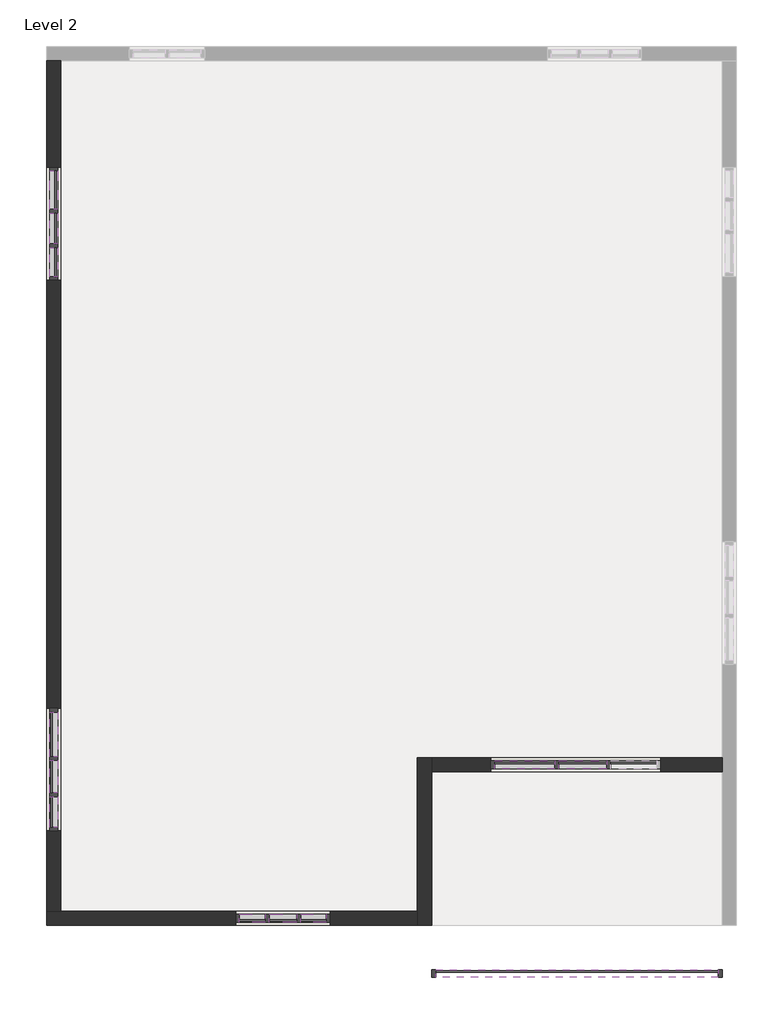
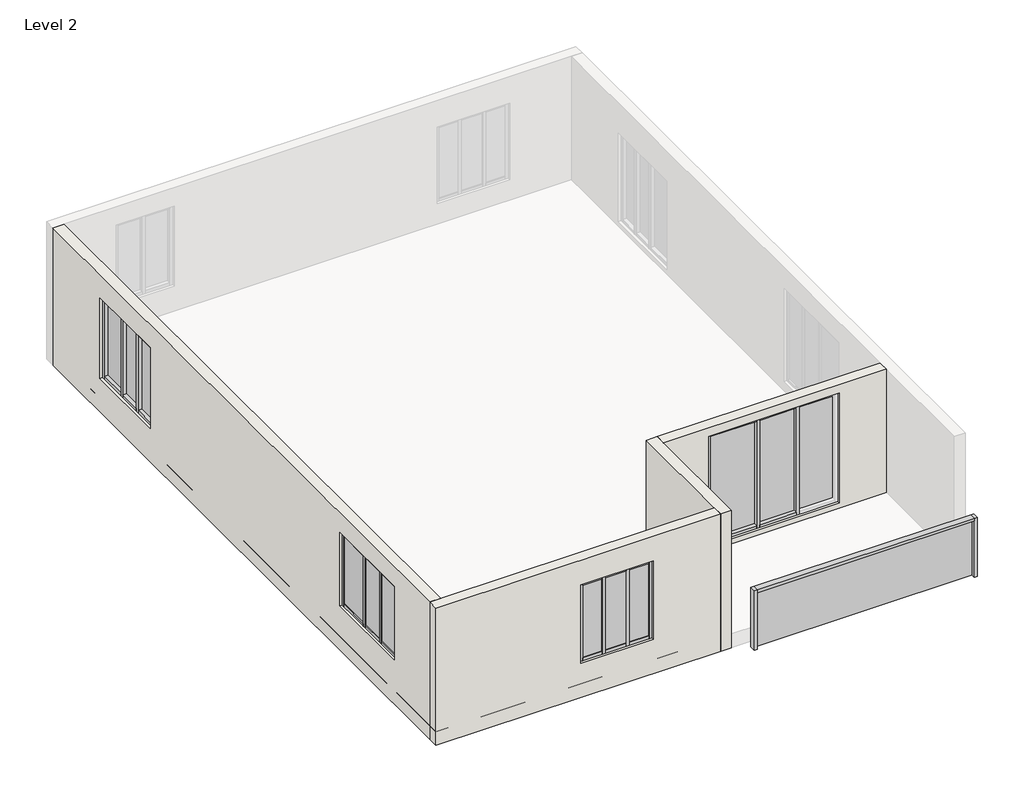
# One storey, part 1 of 2: 40 members, 13 plates, 4 walls.
"""IFC4 building model written with IfcOpenShell, lengths in millimetres."""

from ifc_helpers import new_model, si_unit, frame, origin, place, context, project, spatial, polyline, outline, extrude, faceted_brep, transform, mapped, element, save
from components import member_b9f3750b, member_dc106669, member_3f0e0172, member_8f80d2aa, member_972adede, member_801a2072, member_89a537c7, member_e878716d, member_5535eeb3, member_bc7dbe04, member_2ebf4a73, member_18831802, member_49291f33, member_7007ad49, member_dc48f745, member_f6b14484, member_93c3846a, member_58157355, member_af85eb51, member_d6d4b2c2, system_panel_glazed_d119973b, system_panel_glazed_6af1fae1, system_panel_glazed_479de850, system_panel_glazed_4605dce3, system_panel_glazed_a031bbbc, system_panel_glazed_bb2283f1, system_panel_glazed_6e344361, system_panel_glazed_535565c7, system_panel_glazed_bf89bbd2, system_panel_glazed_12ec074a, system_panel_glazed_49c4d9bd, system_panel_glazed_2b100c62

model = new_model("IFC4")

# Units and contexts
model_context = context("Model", 3, world=origin())
ifc_project = project(units=[si_unit("LENGTHUNIT", "METRE", prefix="MILLI")], contexts=[model_context])

# Site, building, storey
site = spatial("IfcSite", under=ifc_project)
building = spatial("IfcBuilding", under=site)
storey = spatial("IfcBuildingStorey", under=building, Name="Level 2", Elevation=3048.0)

# Members
placement = place(None, origin())
member_shape = member_b9f3750b(model_context)
element("IfcMember", 1, ObjectType="Rectangular Mullion : 2.5\" x 5\" rectangular", at=placement, inside=storey, context=model_context, shape_type="MappedRepresentation", body=[
    mapped(member_shape, transform((-16616.0281629, -12772.5178064, 5658.8694579), x_axis=(0.0, 0.0, 1.0), y_axis=(1.0, 0.0, 0.0), z_axis=(0.0, 1.0, 0.0))),
])
member_2_shape = member_dc106669(model_context)
element("IfcMember", 2, ObjectType="Rectangular Mullion : 2.5\" x 5\" rectangular", at=placement, inside=storey, context=model_context, shape_type="MappedRepresentation", body=[
    mapped(member_2_shape, transform((-12634.5781629, -14734.6678064, 5552.8902612), x_axis=(0.0, 0.0, 1.0), y_axis=(0.0, 1.0, 0.0), z_axis=(-1.0, 0.0, 0.0))),
])
element("IfcMember", 3, ObjectType="Rectangular Mullion : 2.5\" x 5\" rectangular", at=placement, inside=storey, context=model_context, shape_type="MappedRepresentation", body=[
    mapped(member_2_shape, transform((-13618.8281629, -14734.6678064, 5552.8902612), x_axis=(0.0, 0.0, 1.0), y_axis=(0.0, 1.0, 0.0), z_axis=(-1.0, 0.0, 0.0))),
])
element("IfcMember", 4, ObjectType="Rectangular Mullion : 2.5\" x 5\" rectangular", at=placement, inside=storey, context=model_context, shape_type="MappedRepresentation", body=[
    mapped(member_2_shape, transform((-13206.0781629, -14734.6678064, 3807.1716172), x_axis=(0.0, 0.0, -1.0), y_axis=(0.0, 1.0, 0.0), z_axis=(1.0, 0.0, 0.0))),
])
element("IfcMember", 5, ObjectType="Rectangular Mullion : 2.5\" x 5\" rectangular", at=placement, inside=storey, context=model_context, shape_type="MappedRepresentation", body=[
    mapped(member_2_shape, transform((-12221.8281629, -14734.6678064, 3807.1716172), x_axis=(0.0, 0.0, -1.0), y_axis=(0.0, 1.0, 0.0), z_axis=(1.0, 0.0, 0.0))),
])
element("IfcMember", 6, ObjectType="Rectangular Mullion : 2.5\" x 5\" rectangular", at=placement, inside=storey, context=model_context, shape_type="MappedRepresentation", body=[
    mapped(member_shape, transform((-16616.0281629, -13261.4678064, 4022.0249389), x_axis=(0.0, 0.0, -1.0), y_axis=(1.0, 0.0, 0.0), z_axis=(0.0, -1.0, 0.0))),
])
member_3_shape = member_3f0e0172(model_context)
element("IfcMember", 7, ObjectType="Rectangular Mullion : 2.5\" x 5\" rectangular", at=placement, inside=storey, context=model_context, shape_type="MappedRepresentation", body=[
    mapped(member_3_shape, transform((-16616.0281629, -2682.3678064, 3791.862485), x_axis=(0.0, 0.0, -1.0), y_axis=(-1.0, 0.0, 0.0), z_axis=(0.0, 1.0, 0.0))),
])
member_4_shape = member_8f80d2aa(model_context)
element("IfcMember", 8, ObjectType="Rectangular Mullion : 2.5\" x 5\" rectangular", at=placement, inside=storey, context=model_context, shape_type="MappedRepresentation", body=[
    mapped(member_4_shape, transform((-16616.0281629, -12709.0178064, 4022.0249389), x_axis=(0.0, 0.0, -1.0), y_axis=(1.0, 0.0, 0.0), z_axis=(0.0, -1.0, 0.0))),
])
element("IfcMember", 9, ObjectType="Rectangular Mullion : 2.5\" x 5\" rectangular", at=placement, inside=storey, context=model_context, shape_type="MappedRepresentation", body=[
    mapped(member_4_shape, transform((-16616.0281629, -12188.3178064, 5658.8694579), x_axis=(0.0, 0.0, 1.0), y_axis=(1.0, 0.0, 0.0), z_axis=(0.0, 1.0, 0.0))),
])
element("IfcMember", 10, ObjectType="Rectangular Mullion : 2.5\" x 5\" rectangular", at=placement, inside=storey, context=model_context, shape_type="MappedRepresentation", body=[
    mapped(member_3_shape, transform((-16616.0281629, -3298.3178064, 5580.8929613), x_axis=(0.0, 0.0, 1.0), y_axis=(-1.0, 0.0, 0.0), z_axis=(0.0, -1.0, 0.0))),
])
member_5_shape = member_972adede(model_context)
element("IfcMember", 11, ObjectType="Rectangular Mullion : 2.5\" x 5\" rectangular", at=placement, inside=storey, context=model_context, shape_type="MappedRepresentation", body=[
    mapped(member_5_shape, transform((-7694.2781629, -12258.1678064, 5911.9599258), x_axis=(0.0, 0.0, 1.0), y_axis=(0.0, -1.0, 0.0), z_axis=(1.0, 0.0, 0.0))),
])
member_6_shape = member_801a2072(model_context)
element("IfcMember", 12, ObjectType="Rectangular Mullion : 2.5\" x 5\" rectangular", at=placement, inside=storey, context=model_context, shape_type="MappedRepresentation", body=[
    mapped(member_6_shape, transform((-8532.4781629, -12258.1678064, 5911.9599258), x_axis=(0.0, 0.0, 1.0), y_axis=(0.0, -1.0, 0.0), z_axis=(1.0, 0.0, 0.0))),
])
member_7_shape = member_89a537c7(model_context)
element("IfcMember", 13, ObjectType="Rectangular Mullion : 2.5\" x 5\" rectangular", at=placement, inside=storey, context=model_context, shape_type="MappedRepresentation", body=[
    mapped(member_7_shape, transform((-7662.5281629, -12258.1678064, 3466.2078322), x_axis=(1.0, 0.0, 0.0), y_axis=(0.0, -1.0, 0.0), z_axis=(0.0, 0.0, -1.0))),
])
element("IfcMember", 14, ObjectType="Rectangular Mullion : 2.5\" x 5\" rectangular", at=placement, inside=storey, context=model_context, shape_type="MappedRepresentation", body=[
    mapped(member_7_shape, transform((-8500.7281629, -12258.1678064, 3466.2078322), x_axis=(1.0, 0.0, 0.0), y_axis=(0.0, -1.0, 0.0), z_axis=(0.0, 0.0, -1.0))),
])
element("IfcMember", 15, ObjectType="Rectangular Mullion : 2.5\" x 5\" rectangular", at=placement, inside=storey, context=model_context, shape_type="MappedRepresentation", body=[
    mapped(member_5_shape, transform((-8468.9781629, -12258.1678064, 3466.2078322), x_axis=(0.0, 0.0, -1.0), y_axis=(0.0, -1.0, 0.0), z_axis=(-1.0, 0.0, 0.0))),
])
element("IfcMember", 16, ObjectType="Rectangular Mullion : 2.5\" x 5\" rectangular", at=placement, inside=storey, context=model_context, shape_type="MappedRepresentation", body=[
    mapped(member_6_shape, transform((-9504.0281629, -12258.1678064, 3466.2078322), x_axis=(0.0, 0.0, -1.0), y_axis=(0.0, -1.0, 0.0), z_axis=(-1.0, 0.0, 0.0))),
])
member_8_shape = member_e878716d(model_context)
element("IfcMember", 17, ObjectType="Rectangular Mullion : 2.5\" x 5\" rectangular", at=placement, inside=storey, context=model_context, shape_type="MappedRepresentation", body=[
    mapped(member_8_shape, transform((-9567.5281629, -12258.1678064, 5911.9599258), x_axis=(-1.0, 0.0, 0.0), y_axis=(0.0, -1.0, 0.0), z_axis=(0.0, 0.0, 1.0))),
])
member_9_shape = member_5535eeb3(model_context)
element("IfcMember", 18, ObjectType="Rectangular Mullion : 2.5\" x 5\" rectangular", at=placement, inside=storey, context=model_context, shape_type="MappedRepresentation", body=[
    mapped(member_9_shape, transform((-16616.0281629, -3920.6178064, 3791.862485), x_axis=(0.0, 0.0, -1.0), y_axis=(-1.0, 0.0, 0.0), z_axis=(0.0, 1.0, 0.0))),
])
element("IfcMember", 19, ObjectType="Rectangular Mullion : 2.5\" x 5\" rectangular", at=placement, inside=storey, context=model_context, shape_type="MappedRepresentation", body=[
    mapped(member_9_shape, transform((-16616.0281629, -4384.1678064, 5580.8929613), x_axis=(0.0, 0.0, 1.0), y_axis=(-1.0, 0.0, 0.0), z_axis=(0.0, -1.0, 0.0))),
])
member_10_shape = member_bc7dbe04(model_context)
element("IfcMember", 20, ObjectType="Rectangular Mullion : 2.5\" x 5\" rectangular", at=placement, inside=storey, context=model_context, shape_type="MappedRepresentation", body=[
    mapped(member_10_shape, transform((-12698.0781629, -14734.6678064, 3807.1716172), x_axis=(0.0, 0.0, -1.0), y_axis=(0.0, 1.0, 0.0), z_axis=(1.0, 0.0, 0.0))),
])
element("IfcMember", 21, ObjectType="Rectangular Mullion : 2.5\" x 5\" rectangular", at=placement, inside=storey, context=model_context, shape_type="MappedRepresentation", body=[
    mapped(member_10_shape, transform((-13142.5781629, -14734.6678064, 5552.8902612), x_axis=(0.0, 0.0, 1.0), y_axis=(0.0, 1.0, 0.0), z_axis=(-1.0, 0.0, 0.0))),
])
member_11_shape = member_2ebf4a73(model_context)
element("IfcMember", 22, ObjectType="Rectangular Mullion : 2.5\" x 5\" rectangular", at=placement, inside=storey, context=model_context, shape_type="MappedRepresentation", body=[
    mapped(member_11_shape, transform((-16616.0281629, -3857.1178064, 5580.8929613), x_axis=(0.0, 0.0, 1.0), y_axis=(-1.0, 0.0, 0.0), z_axis=(0.0, -1.0, 0.0))),
])
member_12_shape = member_18831802(model_context)
element("IfcMember", 23, ObjectType="Rectangular Mullion : 2.5\" x 5\" rectangular", at=placement, inside=storey, context=model_context, shape_type="MappedRepresentation", body=[
    mapped(member_12_shape, transform((-16616.0281629, -3330.0678064, 3791.862485), x_axis=(0.0, -1.0, 0.0), y_axis=(-1.0, 0.0, 0.0), z_axis=(0.0, 0.0, -1.0))),
])
element("IfcMember", 24, ObjectType="Rectangular Mullion : 2.5\" x 5\" rectangular", at=placement, inside=storey, context=model_context, shape_type="MappedRepresentation", body=[
    mapped(member_12_shape, transform((-16616.0281629, -3888.8678064, 3791.862485), x_axis=(0.0, -1.0, 0.0), y_axis=(-1.0, 0.0, 0.0), z_axis=(0.0, 0.0, -1.0))),
])
element("IfcMember", 25, ObjectType="Rectangular Mullion : 2.5\" x 5\" rectangular", at=placement, inside=storey, context=model_context, shape_type="MappedRepresentation", body=[
    mapped(member_11_shape, transform((-16616.0281629, -3361.8178064, 3791.862485), x_axis=(0.0, 0.0, -1.0), y_axis=(-1.0, 0.0, 0.0), z_axis=(0.0, 1.0, 0.0))),
])
member_13_shape = member_49291f33(model_context)
element("IfcMember", 26, ObjectType="Rectangular Mullion : 2.5\" x 5\" rectangular", at=placement, inside=storey, context=model_context, shape_type="MappedRepresentation", body=[
    mapped(member_13_shape, transform((-16616.0281629, -4447.6678064, 3791.862485), x_axis=(0.0, -1.0, 0.0), y_axis=(-1.0, 0.0, 0.0), z_axis=(0.0, 0.0, -1.0))),
])
element("IfcMember", 27, ObjectType="Rectangular Mullion : 2.5\" x 5\" rectangular", at=placement, inside=storey, context=model_context, shape_type="MappedRepresentation", body=[
    mapped(member_13_shape, transform((-16616.0281629, -2618.8678064, 5580.8929613), x_axis=(0.0, 1.0, 0.0), y_axis=(-1.0, 0.0, 0.0), z_axis=(0.0, 0.0, 1.0))),
])
member_14_shape = member_7007ad49(model_context)
element("IfcMember", 28, ObjectType="Rectangular Mullion : 2.5\" x 5\" rectangular", at=placement, inside=storey, context=model_context, shape_type="MappedRepresentation", body=[
    mapped(member_14_shape, transform((-16616.0281629, -11407.2678064, 5658.8694579), x_axis=(0.0, 0.0, 1.0), y_axis=(1.0, 0.0, 0.0), z_axis=(0.0, 1.0, 0.0))),
])
member_15_shape = member_dc48f745(model_context)
element("IfcMember", 29, ObjectType="Rectangular Mullion : 2.5\" x 5\" rectangular", at=placement, inside=storey, context=model_context, shape_type="MappedRepresentation", body=[
    mapped(member_15_shape, transform((-16616.0281629, -12156.5678064, 4022.0249389), x_axis=(0.0, 1.0, 0.0), y_axis=(1.0, 0.0, 0.0), z_axis=(0.0, 0.0, -1.0))),
])
element("IfcMember", 30, ObjectType="Rectangular Mullion : 2.5\" x 5\" rectangular", at=placement, inside=storey, context=model_context, shape_type="MappedRepresentation", body=[
    mapped(member_15_shape, transform((-16616.0281629, -12740.7678064, 4022.0249389), x_axis=(0.0, 1.0, 0.0), y_axis=(1.0, 0.0, 0.0), z_axis=(0.0, 0.0, -1.0))),
])
element("IfcMember", 31, ObjectType="Rectangular Mullion : 2.5\" x 5\" rectangular", at=placement, inside=storey, context=model_context, shape_type="MappedRepresentation", body=[
    mapped(member_14_shape, transform((-16616.0281629, -12124.8178064, 4022.0249389), x_axis=(0.0, 0.0, -1.0), y_axis=(1.0, 0.0, 0.0), z_axis=(0.0, -1.0, 0.0))),
])
member_16_shape = member_f6b14484(model_context)
element("IfcMember", 32, ObjectType="Rectangular Mullion : 2.5\" x 5\" rectangular", at=placement, inside=storey, context=model_context, shape_type="MappedRepresentation", body=[
    mapped(member_16_shape, transform((-16616.0281629, -13324.9678064, 5658.8694579), x_axis=(0.0, -1.0, 0.0), y_axis=(1.0, 0.0, 0.0), z_axis=(0.0, 0.0, 1.0))),
])
element("IfcMember", 33, ObjectType="Rectangular Mullion : 2.5\" x 5\" rectangular", at=placement, inside=storey, context=model_context, shape_type="MappedRepresentation", body=[
    mapped(member_16_shape, transform((-16616.0281629, -11343.7678064, 4022.0249389), x_axis=(0.0, 1.0, 0.0), y_axis=(1.0, 0.0, 0.0), z_axis=(0.0, 0.0, -1.0))),
])
member_17_shape = member_93c3846a(model_context)
element("IfcMember", 34, ObjectType="Rectangular Mullion : 2.5\" x 5\" rectangular", at=placement, inside=storey, context=model_context, shape_type="MappedRepresentation", body=[
    mapped(member_17_shape, transform((-13174.3281629, -14734.6678064, 3807.1716172), x_axis=(-1.0, 0.0, 0.0), y_axis=(0.0, 1.0, 0.0), z_axis=(0.0, 0.0, -1.0))),
])
element("IfcMember", 35, ObjectType="Rectangular Mullion : 2.5\" x 5\" rectangular", at=placement, inside=storey, context=model_context, shape_type="MappedRepresentation", body=[
    mapped(member_17_shape, transform((-12666.3281629, -14734.6678064, 3807.1716172), x_axis=(-1.0, 0.0, 0.0), y_axis=(0.0, 1.0, 0.0), z_axis=(0.0, 0.0, -1.0))),
])
member_18_shape = member_58157355(model_context)
element("IfcMember", 36, ObjectType="Rectangular Mullion : 2.5\" x 5\" rectangular", at=placement, inside=storey, context=model_context, shape_type="MappedRepresentation", body=[
    mapped(member_18_shape, transform((-13682.3281629, -14734.6678064, 3807.1716172), x_axis=(-1.0, 0.0, 0.0), y_axis=(0.0, 1.0, 0.0), z_axis=(0.0, 0.0, -1.0))),
])
element("IfcMember", 37, ObjectType="Rectangular Mullion : 2.5\" x 5\" rectangular", at=placement, inside=storey, context=model_context, shape_type="MappedRepresentation", body=[
    mapped(member_18_shape, transform((-12158.3281629, -14734.6678064, 5552.8902612), x_axis=(1.0, 0.0, 0.0), y_axis=(0.0, 1.0, 0.0), z_axis=(0.0, 0.0, 1.0))),
])
member_19_shape = member_af85eb51(model_context)
element("IfcMember", 38, ObjectType="Rectangular Mullion : 2.5\" x 5\" rectangular", at=placement, inside=storey, context=model_context, shape_type="MappedRepresentation", body=[
    mapped(member_19_shape, transform((-10520.0281629, -15623.6678064, 4815.0330157), x_axis=(-1.0, 0.0, 0.0), y_axis=(0.0, -1.0, 0.0), z_axis=(0.0, 0.0, 1.0))),
])
member_20_shape = member_d6d4b2c2(model_context)
element("IfcMember", 39, ObjectType="Rectangular Mullion : 2.5\" x 5\" rectangular", at=placement, inside=storey, context=model_context, shape_type="MappedRepresentation", body=[
    mapped(member_20_shape, transform((-5897.2281629, -15623.6678064, 4815.0330157), x_axis=(0.0, 0.0, 1.0), y_axis=(0.0, -1.0, 0.0), z_axis=(1.0, 0.0, 0.0))),
])
element("IfcMember", 40, ObjectType="Rectangular Mullion : 2.5\" x 5\" rectangular", at=placement, inside=storey, context=model_context, shape_type="MappedRepresentation", body=[
    mapped(member_19_shape, transform((-5833.7281629, -15623.6678064, 3499.8590978), x_axis=(1.0, 0.0, 0.0), y_axis=(0.0, -1.0, 0.0), z_axis=(0.0, 0.0, -1.0))),
])

# Plates
system_panel_glazed_shape = system_panel_glazed_d119973b(model_context)
element("IfcPlate", 41, ObjectType="System Panel : Glazed", at=placement, inside=storey, context=model_context, shape_type="MappedRepresentation", body=[
    mapped(system_panel_glazed_shape, transform((-9018.2531629, -12258.1678064, 3529.7078322), x_axis=(1.0, 0.0, 0.0), y_axis=(0.0, 1.0, 0.0), z_axis=(0.0, 0.0, 1.0))),
])
system_panel_glazed_2_shape = system_panel_glazed_6af1fae1(model_context)
element("IfcPlate", 42, ObjectType="System Panel : Glazed", at=placement, inside=storey, context=model_context, shape_type="MappedRepresentation", body=[
    mapped(system_panel_glazed_2_shape, transform((-8081.6281629, -12258.1678064, 3529.7078322), x_axis=(1.0, 0.0, 0.0), y_axis=(0.0, 1.0, 0.0), z_axis=(0.0, 0.0, 1.0))),
])
system_panel_glazed_3_shape = system_panel_glazed_479de850(model_context)
element("IfcPlate", 43, ObjectType="System Panel : Glazed", at=placement, inside=storey, context=model_context, shape_type="MappedRepresentation", body=[
    mapped(system_panel_glazed_3_shape, transform((-7259.3031629, -12258.1678064, 3529.7078322), x_axis=(1.0, 0.0, 0.0), y_axis=(0.0, 1.0, 0.0), z_axis=(0.0, 0.0, 1.0))),
])
system_panel_glazed_4_shape = system_panel_glazed_4605dce3(model_context)
element("IfcPlate", 44, ObjectType="System Panel : Glazed", at=placement, inside=storey, context=model_context, shape_type="MappedRepresentation", body=[
    mapped(system_panel_glazed_4_shape, transform((-16616.0281629, -2990.3428064, 3855.362485), x_axis=(0.0, -1.0, 0.0), y_axis=(1.0, 0.0, 0.0), z_axis=(0.0, 0.0, 1.0))),
])
system_panel_glazed_5_shape = system_panel_glazed_a031bbbc(model_context)
element("IfcPlate", 45, ObjectType="System Panel : Glazed", at=placement, inside=storey, context=model_context, shape_type="MappedRepresentation", body=[
    mapped(system_panel_glazed_5_shape, transform((-16616.0281629, -3609.4678064, 3855.362485), x_axis=(0.0, -1.0, 0.0), y_axis=(1.0, 0.0, 0.0), z_axis=(0.0, 0.0, 1.0))),
])
system_panel_glazed_6_shape = system_panel_glazed_bb2283f1(model_context)
element("IfcPlate", 46, ObjectType="System Panel : Glazed", at=placement, inside=storey, context=model_context, shape_type="MappedRepresentation", body=[
    mapped(system_panel_glazed_6_shape, transform((-16616.0281629, -4152.3928064, 3855.362485), x_axis=(0.0, -1.0, 0.0), y_axis=(1.0, 0.0, 0.0), z_axis=(0.0, 0.0, 1.0))),
])
system_panel_glazed_7_shape = system_panel_glazed_6e344361(model_context)
element("IfcPlate", 47, ObjectType="System Panel : Glazed", at=placement, inside=storey, context=model_context, shape_type="MappedRepresentation", body=[
    mapped(system_panel_glazed_7_shape, transform((-16616.0281629, -13016.9928064, 4085.5249389), x_axis=(0.0, 1.0, 0.0), y_axis=(-1.0, 0.0, 0.0), z_axis=(0.0, 0.0, 1.0))),
])
system_panel_glazed_8_shape = system_panel_glazed_535565c7(model_context)
element("IfcPlate", 48, ObjectType="System Panel : Glazed", at=placement, inside=storey, context=model_context, shape_type="MappedRepresentation", body=[
    mapped(system_panel_glazed_8_shape, transform((-16616.0281629, -11766.0428064, 4085.5249389), x_axis=(0.0, 1.0, 0.0), y_axis=(-1.0, 0.0, 0.0), z_axis=(0.0, 0.0, 1.0))),
])
system_panel_glazed_9_shape = system_panel_glazed_bf89bbd2(model_context)
element("IfcPlate", 49, ObjectType="System Panel : Glazed", at=placement, inside=storey, context=model_context, shape_type="MappedRepresentation", body=[
    mapped(system_panel_glazed_9_shape, transform((-16616.0281629, -12448.6678064, 4085.5249389), x_axis=(0.0, 1.0, 0.0), y_axis=(-1.0, 0.0, 0.0), z_axis=(0.0, 0.0, 1.0))),
])
system_panel_glazed_10_shape = system_panel_glazed_12ec074a(model_context)
element("IfcPlate", 50, ObjectType="System Panel : Glazed", at=placement, inside=storey, context=model_context, shape_type="MappedRepresentation", body=[
    mapped(system_panel_glazed_10_shape, transform((-12428.2031629, -14734.6678064, 3870.6716172), x_axis=(-1.0, 0.0, 0.0), y_axis=(0.0, -1.0, 0.0), z_axis=(0.0, 0.0, 1.0))),
])
element("IfcPlate", 51, ObjectType="System Panel : Glazed", at=placement, inside=storey, context=model_context, shape_type="MappedRepresentation", body=[
    mapped(system_panel_glazed_10_shape, transform((-13412.4531629, -14734.6678064, 3870.6716172), x_axis=(-1.0, 0.0, 0.0), y_axis=(0.0, -1.0, 0.0), z_axis=(0.0, 0.0, 1.0))),
])
system_panel_glazed_11_shape = system_panel_glazed_49c4d9bd(model_context)
element("IfcPlate", 52, ObjectType="System Panel : Glazed", at=placement, inside=storey, context=model_context, shape_type="MappedRepresentation", body=[
    mapped(system_panel_glazed_11_shape, transform((-12920.3281629, -14734.6678064, 3870.6716172), x_axis=(-1.0, 0.0, 0.0), y_axis=(0.0, -1.0, 0.0), z_axis=(0.0, 0.0, 1.0))),
])
system_panel_glazed_12_shape = system_panel_glazed_2b100c62(model_context)
element("IfcPlate", 53, ObjectType="System Panel : Glazed", at=placement, inside=storey, context=model_context, shape_type="MappedRepresentation", body=[
    mapped(system_panel_glazed_12_shape, transform((-8176.8781629, -15623.6678064, 3499.8590978), x_axis=(1.0, 0.0, 0.0), y_axis=(0.0, 1.0, 0.0), z_axis=(0.0, 0.0, 1.0))),
])

# Walls
element("IfcWall", 54, ObjectType="9\"", at=placement, inside=storey, context=model_context, shape_type="Brep", body=[
    faceted_brep([(-10748.6281629, -12143.8678064, 3048.0), (-10748.6281629, -14620.3678064, 3048.0), (-10748.6281629, -14848.9678064, 3048.0), (-10748.6281629, -14848.9678064, 6096.0), (-10748.6281629, -14620.3678064, 6096.0), (-10748.6281629, -12143.8678064, 6096.0), (-10520.0281629, -12143.8678064, 3048.0), (-10520.0281629, -12143.8678064, 6096.0), (-10520.0281629, -12372.4678064, 6096.0), (-10520.0281629, -14848.9678064, 6096.0), (-10520.0281629, -14848.9678064, 3048.0), (-10520.0281629, -12372.4678064, 3048.0)], [[[0, 1, 2, 3, 4, 5]], [[6, 7, 8, 9, 10, 11]], [[2, 1, 0, 6, 11, 10]], [[5, 4, 3, 9, 8, 7]], [[3, 2, 10, 9]], [[0, 5, 7, 6]]]),
])
element("IfcWall", 55, ObjectType="9\"", at=placement, inside=storey, context=model_context, shape_type="Brep", body=[
    faceted_brep([(-10748.6281629, -14620.3678064, 3048.0), (-16501.7281629, -14620.3678064, 3048.0), (-16730.3281629, -14620.3678064, 3048.0), (-16730.3281629, -14620.3678064, 6096.0), (-16501.7281629, -14620.3678064, 6096.0), (-10748.6281629, -14620.3678064, 6096.0), (-12158.3281629, -14620.3678064, 3807.1716172), (-12158.3281629, -14620.3678064, 5552.8902612), (-13682.3281629, -14620.3678064, 5552.8902612), (-13682.3281629, -14620.3678064, 3807.1716172), (-16730.3281629, -14848.9678064, 3048.0), (-10748.6281629, -14848.9678064, 3048.0), (-10748.6281629, -14848.9678064, 6096.0), (-16730.3281629, -14848.9678064, 6096.0), (-12158.3281629, -14848.9678064, 5552.8902612), (-12158.3281629, -14848.9678064, 3807.1716172), (-13682.3281629, -14848.9678064, 3807.1716172), (-13682.3281629, -14848.9678064, 5552.8902612)], [[[0, 1, 2, 3, 4, 5], [6, 7, 8, 9]], [[10, 11, 12, 13], [14, 15, 16, 17]], [[2, 1, 0, 11, 10]], [[5, 4, 3, 13, 12]], [[0, 5, 12, 11]], [[3, 2, 10, 13]], [[6, 15, 14, 7]], [[7, 14, 17, 8]], [[8, 17, 16, 9]], [[15, 6, 9, 16]]]),
])
element("IfcWall", 56, ObjectType="9\"", at=placement, inside=storey, context=model_context, shape_type="SweptSolid", body=[
    extrude(outline(polyline([(-904.3678064, 3048.0), (-14620.3678064, 3048.0), (-14620.3678064, 6096.0), (-904.3678064, 6096.0), (-904.3678064, 3048.0)]), holes=[polyline([(-2618.8678064, 3791.862485), (-2618.8678064, 5580.8929613), (-4447.6678064, 5580.8929613), (-4447.6678064, 3791.862485), (-2618.8678064, 3791.862485)]), polyline([(-13324.9678064, 5658.8694579), (-13324.9678064, 4022.0249389), (-11343.7678064, 4022.0249389), (-11343.7678064, 5658.8694579), (-13324.9678064, 5658.8694579)])]), frame((-16730.3281629, 0.0, 0.0), z_axis=(1.0, 0.0, 0.0), x_axis=(0.0, 1.0, 0.0)), (0.0, 0.0, 1.0), 228.6),
])
element("IfcWall", 57, ObjectType="9\"", at=placement, inside=storey, context=model_context, shape_type="SweptSolid", body=[
    extrude(outline(polyline([(3048.0, -10520.0281629), (3048.0, -5833.7281629), (6096.0, -5833.7281629), (6096.0, -10520.0281629), (3048.0, -10520.0281629)]), holes=[polyline([(3466.2078322, -9567.5281629), (5911.9599258, -9567.5281629), (5911.9599258, -6824.3281629), (3466.2078322, -6824.3281629), (3466.2078322, -9567.5281629)])]), frame((0.0, -12372.4678064, 0.0), z_axis=(0.0, 1.0, 0.0), x_axis=(0.0, 0.0, 1.0)), (0.0, 0.0, 1.0), 228.6),
])

save(model, "model.ifc")

# Revit data of these elements
# Type "Rectangular Mullion : 2.5\" x 5\" rectangular"
#   built-in parameter 1007304 = 0.416667 (stored number, unit not read)
#   built-in parameter 1007301 = 0.104167 (stored number, unit not read)
#   built-in parameter 1007300 = 0.104167 (stored number, unit not read)
# Type "System Panel : Glazed"
#   Construction Type Id = "GSP4R"
#   Analytic Construction = "1/8 in Pilkington single glazing"
#   Visual Light Transmittance = 0.9
#   Solar Heat Gain Coefficient = 0.86
#   Heat Transfer Coefficient (U) = 1.18115 BTU/(h·ft²·°F)
#   Define Thermal Properties by = 1
# Type "9\""
#   Assembly Code = "B2010"
#   Layers, outside or top first: 0' - 9" no material (function 1)
# Elements 1, 2, 3, 4, 5, 6, 7, 8, 9, 10, 11, 12, 13, 14, 15, 16, 17, 18, 19, 20, 21, 22, 23, 24, 25, 26, 27, 28, 29, 30, 31, 32, 33, 34, 35, 36, 37, 38, 39, 40 (IfcMember, "Rectangular Mullion : 2.5\" x 5\" rectangular")
#   Phase Created = New Construction
#   Materials on its faces: "Aluminum"
# Elements 41, 42, 43, 44, 45, 46, 47, 48, 49, 50, 51, 52, 53 (IfcPlate, "System Panel : Glazed")
#   Phase Created = New Construction
#   Materials on its faces: "Glass"
# Elements 54, 55, 56, 57 (IfcWall, "9\"")
#   Top Offset = 0' - 0"
#   Base Offset = 0' - 0"
#   Unconnected Height = 10' - 0"
#   wall height = 10' - 0"
#   Phase Created = New Construction
#   Base Constraint = Level 2
#   Materials on its faces: "Default Wall"
# Materials
#   "Aluminum": class "Metal", colour RGB 247 247 247, transparency 0, Description = "Aluminum 6061", Cost = 0
#   "Glass": class "Glass", colour RGB 0 128 192, transparency 0.75, Description = "Soda Lime Glass", Cost = 0
#   "Default Wall": colour RGB 128 128 128, transparency 0, Cost = 0
